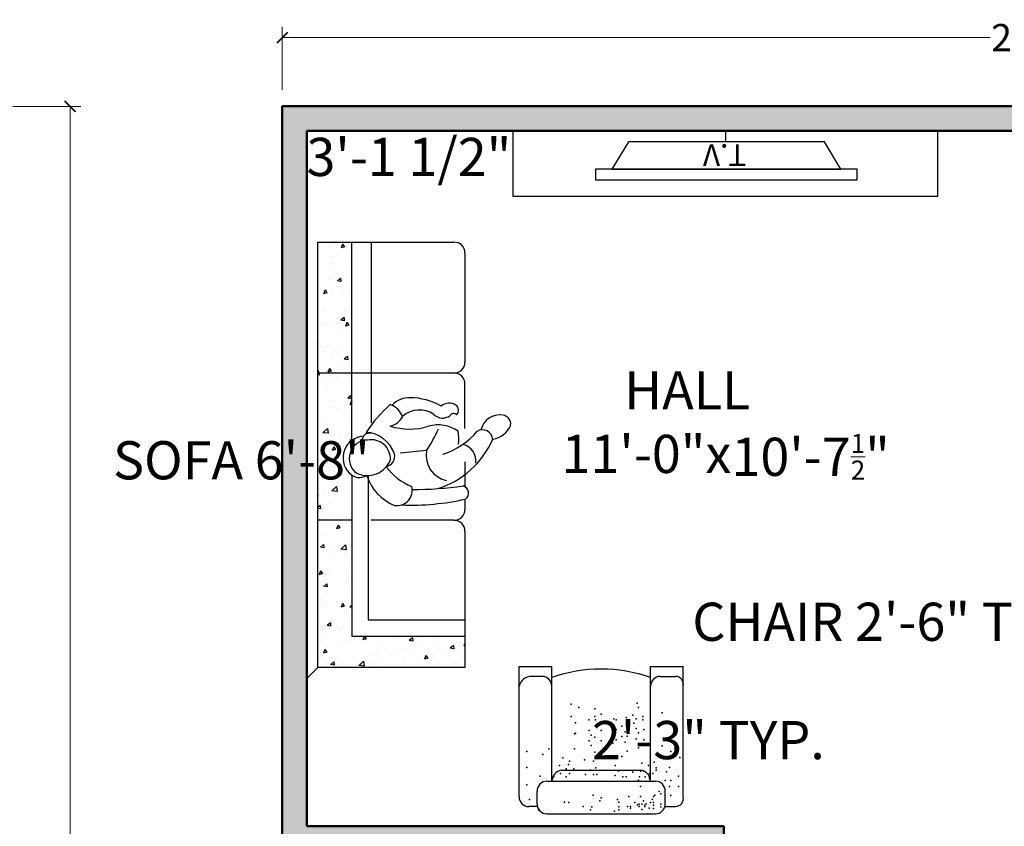
# Model space of a CAD drawing. Units: inches. Extents: x 4508 to 5907, y 877 to 1592.
# Tile 16 of 20: x 5203 to 5383, y 1443 to 1591. Entities that reach past the tile are written whole.
import ezdxf

# ---------------------------------------------------------------- set-up
doc = ezdxf.new("R2010")
doc.units = ezdxf.units.IN
doc.layers.get('DEFPOINTS').update_dxf_attribs({"color": 8})
for name, color, linetype, lineweight in [('A-ANNO-DIMS', 2, 'Continuous', 18), ('A-FURN', 24, 'Continuous', 18), ('A-WALL', 7, 'Continuous', 50), ('A-WALL-PATT', 8, 'Continuous', 13)]:
    doc.layers.add(name, color=color, linetype=linetype, lineweight=lineweight)
doc.layers.add('doors & windows', color=30, linetype='Continuous')
doc.layers.add('furniture', color=24, linetype='Continuous')
doc.styles.get("Standard").update_dxf_attribs({"font": 'arial.ttf'})
doc.dimstyles.new('details', dxfattribs={"dimtxt": 5, "dimasz": 2, "dimexe": 2, "dimexo": 3, "dimgap": 1, "dimtad": 0, "dimdec": 1, "dimzin": 0, "dimdsep": 46, "dimlunit": 4, "dimtxsty": 'Standard', "dimblk": 'ARCHTICK', "dimcen": 3, "dimclrd": 256, "dimclre": 256, "dimclrt": 256, "dimadec": 0, "dimazin": 0, "dimtfac": 0.5, "dimtdec": 1, "dimtofl": 0, "dimtmove": 0, "dimatfit": 3, "dimldrblk": 'CLOSEDBLANK', "dimfxl": 2, "dimtolj": 1, "dimtzin": 0, "dimlwd": -1, "dimlwe": -1, "dimarcsym": 0})
doc.dimstyles.new('text', dxfattribs={"dimtxt": 7, "dimasz": 0, "dimexe": 3, "dimexo": 3, "dimgap": 0, "dimtad": 1, "dimtih": 1, "dimtoh": 1, "dimzin": 3, "dimdsep": 46, "dimlunit": 4, "dimtxsty": 'Standard', "dimblk": 'CLOSEDBLANK', "dimcen": 3, "dimse1": 1, "dimse2": 1, "dimsd1": 1, "dimsd2": 1, "dimclrd": 256, "dimclre": 256, "dimclrt": 256, "dimadec": 0, "dimazin": 0, "dimtfac": 0.5, "dimtofl": 0, "dimtmove": 0, "dimatfit": 3, "dimfxl": 3, "dimtolj": 1, "dimtzin": 0, "dimlwd": -1, "dimlwe": -1, "dimarcsym": 0})

# ---------------------------------------------------------------- blocks, each defined once
blk = doc.blocks.new('_ArchTick')
at = {"color": 0, "linetype": 'ByBlock', "const_width": 0.15}
blk.add_lwpolyline([(-0.5, -0.5), (0.5, 0.5)], dxfattribs=at)
blk = doc.blocks.new('*D77')
at = {"layer": 'A-ANNO-DIMS', "color": 0, "transparency": 16777216}
for p, q in [((5201.49, 1574.7), (5213.97, 1574.7)), ((5211.97, 1574.7), (5211.97, 1255.95)), ((5211.97, 926.7), (5211.97, 1245.46)), ((5201.49, 926.7), (5213.97, 926.7))]:
    blk.add_line(p, q, dxfattribs=at)
at = {"layer": 'DEFPOINTS', "color": 0, "transparency": 16777216}
for p in [(5198.49, 1574.7), (5211.97, 1574.7), (5198.49, 926.7)]:
    blk.add_point(p, dxfattribs=at)
at = {"layer": 'A-ANNO-DIMS', "color": 0, "transparency": 16777216, "xscale": 2, "yscale": 2, "zscale": 2}
for p, rotation in [((5211.97, 1574.7), 90), ((5211.97, 926.7), 270)]:
    blk.add_blockref('_ArchTick', p, dxfattribs=dict(at, rotation=rotation))
at = {"layer": 'A-ANNO-DIMS', "color": 0, "transparency": 16777216, "insert": (5211.97, 1250.7), "char_height": 5, "attachment_point": 5, "rotation": 90}
blk.add_mtext("\\A1;54'", dxfattribs=at)
blk = doc.blocks.new('_ClosedBlank')
at = {"color": 0, "lineweight": -2}
for p, q in [((-1, 0.167), (0, 0)), ((-1, 0.167), (-1, -0.167)), ((0, 0), (-1, -0.167))]:
    blk.add_line(p, q, dxfattribs=at)
blk = doc.blocks.new('MAN')
at = {"layer": 'doors & windows'}
blk.add_line((1.3, -9.85), (0.89, -5.45), dxfattribs=at)
for centre, radius, start, end in [((0.1, 0.48), 3.6, 2.8928, 134.5528), ((-0.81, 1.3), 2.37, 132.7993, 210.1219), ((1.3, 0.05), 4.16, 155.2349, 248.5051), ((0, 0), 3.06, 359.7942, 144.0351), ((-0.36, -7.56), 8.07, 108.0153, 157.5724), ((-0.98, 0.55), 5.34, 289.2819, 356.6237), ((2.86, -0.44), 1.38, 352.7443, 87.7525), ((-8.99, -19.77), 24.04, 41.647, 56.3067), ((-0.1, -0.61), 3.22, 267.7788, 10.6507), ((4.14, -10.82), 9.46, 125.6851, 158.6987), ((0.38, -2.75), 1.79, 192.3382, 283.0231), ((-5.32, -4.92), 2.54, 170.002, 284.7527), ((15.87, -7.04), 10.97, 162.7002, 196.7262), ((8.59, -3.01), 3.29, 193.5598, 239.9446), ((5.83, -2.73), 3.32, 289.6374, 341.2911), ((6.12, -7.03), 4.01, 358.2671, 46.939), ((34.75, -7.19), 42.53, 177.9613, 192.4551), ((3.84, -8.67), 4.24, 325.4363, 41.8446), ((54.76, -7.35), 59.95, 180.1044, 188.2297), ((-0.78, -6.94), 10.91, 330.7562, 358.8997), ((0.5, -14.05), 4.27, 79.2575, 168.509), ((16.49, 13.41), 27.78, 236.8487, 245.427), ((-0.19, -11.81), 5.78, 325.2412, 16.1794), ((8.85, -12.54), 2.12, 136.0875, 215.1077), ((9.03, -7.36), 14.72, 197.1765, 246.7641), ((12.84, -8.62), 12.77, 197.9012, 229.3504), ((7.06, -13.61), 2.15, 328.4119, 38.6474), ((6.8, -14.37), 0.689, 315.9836, 61.7947), ((8.05, -14.12), 1.05, 224.0636, 323.687), ((-5.78, -15.61), 1.25, 217.214, 345.0614), ((-0.4, -15.27), 2.81, 261.6005, 345.5998), ((3.21, -8.72), 6.53, 262.8142, 281.931), ((3.09, -19.2), 1.68, 274.444, 31.8659), ((4.09, -22.01), 3.16, 349.15, 77.9716), ((6.99, -20.36), 3.8, 187.9766, 248.0432), ((5.75, -22.44), 1.45, 262.6631, 353.5986)]:
    blk.add_arc(centre, radius, start, end, dxfattribs=at)
blk = doc.blocks.new('sofa 2')
at = {"layer": 'furniture', "ltscale": 0.5}
h = blk.add_hatch(dxfattribs=at)
h.set_pattern_fill('AR-CONC', color=256, angle=450, style=0)
h.set_pattern_definition([(40, (-1099.1507, 871.655), (-0.627521, 7.172602), [0.75, -8.25]), (95, (-1099.151, 871.655), (7.52192, -1.387513), [0.6, -6.6]), (349.5486, (-1099.203, 872.253), (6.894395, 5.785094), [0.637402, -7.01142]), (43.8158, (-1097.151, 871.655), (-1.65519, 10.67241), [1.125, -12.375]), (353.3644, (-1097.289, 872.544), (9.74118, 9.34663), [0.9561, -10.51713]), (98.8158, (-1097.151, 871.655), (9.74119, 9.34662), [0.9, -9.9]), (69, (-1097.6507, 872.655), (-4.02619, 5.96907), [0.75, -8.25]), (124, (-1097.651, 872.655), (7.2515, 2.433153), [0.6, -6.6]), (18.5486, (-1097.986, 873.1524), (3.225305, 8.402226), [0.637402, -7.01142]), (52.5, (-1099.1507, 871.655), (3.3289385, 0.1215986), [0, -6.52, 0, -6.7, 0, -6.625]), (82.5, (-1099.1507, 871.655), (3.944117, 2.630695), [0, -3.82, 0, -6.37, 0, -2.525]), (122.5, (-1099.1507, 869.425), (-0.2255487, 5.3382244), [0, -2.5, 0, -7.8, 0, -10.35]), (132.5, (-1099.1507, 868.425), (1.00105, 5.831862), [0, -3.25, 0, -5.18, 0, -7.35])])
h.paths.add_polyline_path([(-8.27, -37.7, 0.168872), (-7.9, -36.76, 0.613808), (-6.95, -30.77, 0.074869), (-8.27, -30.38), (-8.27, -29), (-2, -29), (-2, -56), (-8.27, -56)])
h.paths.add_polyline_path([(-8.27, -7.77), (-29, -7.77), (-29, -2), (-2, -2), (-2, -29), (-8.27, -29)])
h.paths.add_polyline_path([(-8.27, -80), (-2, -80), (-2, -56), (-8.27, -56)])
at = {"layer": 'furniture'}
for p, q in [((-2, -2), (0, 0)), ((-29, -2), (-2, -2)), ((-29, -27), (-29, -2)), ((-2, -2), (-2, -80)), ((-8.27, -7.77), (-29, -7.77)), ((-8.27, -37.27), (-8.27, -7.77)), ((-11.27, -10.77), (-29, -10.77)), ((-11.27, -37.27), (-11.27, -10.77)), ((-27, -29), (-11.8, -29)), ((-8.27, -29), (-2, -29)), ((-29, -32.87), (-29, -31)), ((-29, -39.74), (-29, -35.16)), ((-8.27, -37.7), (-8.27, -37.7)), ((-8.27, -43.66), (-8.27, -80)), ((-29, -45.8), (-29, -54)), ((-11.8, -80), (-11.8, -46.89)), ((-27, -56), (-2, -56)), ((-29, -78), (-29, -58)), ((-2, -80), (-27, -80))]:
    blk.add_line(p, q, dxfattribs=at)
for centre, start, end in [((-27, -27), 180, 270), ((-27, -31), 90, 180), ((-27, -54), 180, 270), ((-27, -58), 90, 180), ((-27, -78), 180, 270)]:
    blk.add_arc(centre, 2, start, end, dxfattribs=at)
at = {"xscale": 1.099999999999999, "yscale": 1.099999999999999, "zscale": 1.099999999999999, "rotation": 270}
blk.add_blockref('MAN', (-11.13, -40.34), dxfattribs=at)
blk = doc.blocks.new('*D82')
at = {"layer": 'DEFPOINTS', "color": 0, "transparency": 16777216}
for p in [(5255.4, 1510.81), (5387.4, 1507.41), (5387.4, 1493.7)]:
    blk.add_point(p, dxfattribs=at)
at = {"layer": 'A-ANNO-DIMS', "color": 0, "transparency": 16777216, "insert": (5317.71, 1516.81), "char_height": 7, "width": 116.2892, "attachment_point": 5}
blk.add_mtext('\\A1;       HALL\\P11\'-0"x', dxfattribs=at)
blk = doc.blocks.new('*D83')
at = {"layer": 'DEFPOINTS', "color": 0, "transparency": 16777216}
for p in [(5332.19, 1570.2), (5347.84, 1570.2), (5313.91, 1442.7)]:
    blk.add_point(p, dxfattribs=at)
at = {"layer": 'A-ANNO-DIMS', "color": 0, "transparency": 16777216, "insert": (5347.84, 1510.45), "char_height": 7, "attachment_point": 5}
blk.add_mtext('\\A1;10\'-7{\\H0.5x;\\S1/2;}"', dxfattribs=at)
blk = doc.blocks.new('tv')
at = {"layer": 'furniture'}
blk.add_line((0, 0), (2, 0), dxfattribs=at)
for points in [[(0, -39), (12, -39), (12, 39), (0, 39)], [(7, 24.19), (7, -23.81), (9, -23.81), (9, 24.19), (7, 24.19)]]:
    blk.add_lwpolyline(points, dxfattribs=at)
blk.add_lwpolyline([(7, -20.81), (7, 21.19), (2, 18.19), (2, -17.81)], close=True, dxfattribs=at)
blk.add_text('T.V', height=4, rotation=270, dxfattribs=at).set_placement((2.46, 3.81))
blk = doc.blocks.new('sofa')
at = {"layer": 'furniture'}
for p, q in [((3.13, 15.05), (27, 15.05)), ((27, 15.05), (27, 9.05)), ((1.33, 11.75), (1.33, 13.25)), ((25.2, 10.85), (25.2, 12.75)), ((1.8, 11.75), (4.13, 11.75)), ((0, 9.95), (0, -9.95)), ((6, 9.95), (6, -9.95)), ((6, 9.05), (27, 9.05)), ((8, 7.25), (8, -7.25)), ((8, 4.04), (8, 3.89)), ((6.03, -9.05), (27, -9.05)), ((27, -9.05), (27, -15.05)), ((1.33, -11.75), (1.33, -13.65)), ((1.8, -11.75), (4.13, -11.75)), ((25.2, -10.85), (25.2, -13.65)), ((3.13, -15.05), (27, -15.05))]:
    blk.add_line(p, q, dxfattribs=at)
for centre, radius, start, end in [((3.13, 13.25), 1.8, 90, 180), ((22.91, 12.82), 2.29, 358.3453, 77.7487), ((1.8, 9.95), 1.8, 90, 180), ((1.8, 9.95), 1.8, 90, 180), ((4.14, 9.89), 1.86, 1.747, 90.2901), ((4.14, 9.89), 1.86, 1.747, 90.2901), ((23.4, 10.85), 1.8, 270, 0), ((5.91, 6.93), 2.12, 8.589, 87.4366), ((-0.79, 0), 27.33, 340.6621, 19.3379), ((5.96, -6.99), 2.06, 272.0036, 352.7589), ((1.8, -9.95), 1.8, 180, 270), ((4.14, -9.89), 1.86, 269.7099, 358.253), ((23.4, -10.85), 1.8, 0, 90), ((2.83, -13.59), 1.5, 182.4941, 281.7559), ((23.7, -13.59), 1.5, 258.2441, 357.5059)]:
    blk.add_arc(centre, radius, start, end, dxfattribs=at)
for p in [(2.64, 13.13), (5.3, 13.66), (8.48, 13.66), (11.4, 13.66), (0.72, 11.51), (6.89, 11.2), (10.87, 10.67), (11.93, 9.61), (6.8, 8.68), (7.42, 7.45), (8.85, 7.66), (2.09, 5.95), (2.11, 6.75), (6.8, 6.43), (7.42, 5.82), (8.24, 6.43), (9.05, 6.02), (9.67, 5.82), (10.28, 7.04), (17.83, 5.52), (20.08, 5.52), (8.24, 5), (11.92, 4.9), (14.64, 4.9), (14.78, 4.7), (16.69, 4.7), (19.47, 4.09), (0.72, 1.97), (1.32, 3.3), (7.21, 2.86), (8.03, 2.04), (9.87, 3.06), (12.53, 1.84), (13.35, 2.21), (14.44, 1.84), (15.26, 2.21), (17.21, 2.25), (1.3, 1.71), (2.38, 0.24), (3.44, 1.44), (7.21, 1.39), (7.21, 0.82), (8.44, 0.98), (9.67, 1.43), (10.49, 0.98), (11.31, 1.19), (13.35, 0.01), (14.03, 1.19), (15.26, 0.01), (17.24, 1.02), (17.85, 1.19), (19.26, 1.19), (2.91, -0.01), (18.24, -0.03), (0.5, -2.45), (0.72, -3.25), (1.26, -3.25), (2.11, -3.25), (2.64, -2.98), (7.01, -2.55), (7.83, -3.16), (8.85, -2.55), (12.94, -2.14), (13.56, -2.75), (14.85, -2.14), (15.46, -2.75), (17.21, -2.75), (17.44, -2.34), (1.03, -5.36), (1.32, -5.36), (1.36, -4.83), (3.17, -5.1), (6.8, -3.98), (6.8, -4.59), (10.49, -3.77), (11.51, -4.79), (13.15, -4.38), (14.17, -3.77), (14.23, -4.79), (15.05, -4.38), (16.07, -3.77), (16.8, -4.79), (17.65, -4.59), (1.36, -6.95), (1.62, -6.69), (1.79, -6.95), (2.05, -6.16), (3.17, -7.22), (5.03, -7.22), (6.19, -6.84), (6.8, -7.04), (7.62, -5.82), (12.12, -6.84), (13.76, -6.43), (14.85, -6.84), (15.66, -6.43), (16.6, -6.02), (17.44, -6.43), (18.06, -5.82), (19.47, -6.84), (20.28, -6.63), (-0.03, -8.54), (0.77, -7.48), (1.03, -8.81), (1.36, -8.01), (1.56, -8.01), (1.79, -7.48), (1.85, -8.28), (2.38, -7.75), (6.39, -8.88), (6.8, -8.06), (7.42, -8.88), (7.83, -7.25), (7.83, -7.86), (8.85, -8.68), (9.26, -7.45), (13.56, -7.86), (15.46, -7.86), (17.24, -7.65), (17.83, -7.65), (0.99, -9.6), (1.58, -9.6), (2.05, -9.07), (2.09, -9.6), (2.64, -9.34), (3.17, -9.6), (3.44, -9.87), (4.09, -10.66), (7.42, -9.49), (8.03, -10.11), (8.44, -10.11), (9.46, -9.7), (1.3, -10.93), (1.79, -10.93), (3.64, -10.93), (5.03, -12.52), (6.09, -11.72), (7.69, -11.99), (8.48, -12.52), (12.46, -11.19), (18.51, -11.19), (3.38, -12.78), (5.03, -14.17), (6.09, -12.78), (6.89, -14.17), (10.34, -14.44), (11.4, -12.78)]:
    blk.add_point(p, dxfattribs=at)
blk = doc.blocks.new('*D112')
at = {"layer": 'A-ANNO-DIMS', "color": 0, "transparency": 16777216}
for p, q in [((5250.9, 1577.7), (5250.9, 1589.3)), ((5529.9, 1577.7), (5529.9, 1589.3)), ((5250.9, 1587.3), (5380.77, 1587.3)), ((5529.9, 1587.3), (5400.03, 1587.3))]:
    blk.add_line(p, q, dxfattribs=at)
at = {"layer": 'DEFPOINTS', "color": 0, "transparency": 16777216}
for p in [(5529.9, 1587.3), (5250.9, 1574.7), (5529.9, 1574.7)]:
    blk.add_point(p, dxfattribs=at)
at = {"layer": 'A-ANNO-DIMS', "color": 0, "transparency": 16777216, "xscale": 2, "yscale": 2, "zscale": 2, "rotation": 180}
blk.add_blockref('_ArchTick', (5250.9, 1587.3), dxfattribs=at)
at = {"layer": 'A-ANNO-DIMS', "color": 0, "transparency": 16777216, "xscale": 2, "yscale": 2, "zscale": 2}
blk.add_blockref('_ArchTick', (5529.9, 1587.3), dxfattribs=at)
at = {"layer": 'A-ANNO-DIMS', "color": 0, "transparency": 16777216, "insert": (5390.4, 1587.3), "char_height": 5, "attachment_point": 5}
blk.add_mtext('\\A1;23\'-3"', dxfattribs=at)
blk = doc.blocks.new('*D174')
at = {"layer": 'DEFPOINTS', "color": 0, "transparency": 16777216}
for p in [(5294.35, 1476.58), (5294.35, 1472.05), (5324.54, 1472.05)]:
    blk.add_point(p, dxfattribs=at)
at = {"layer": 'A-ANNO-DIMS', "transparency": 16777216, "insert": (5362.41, 1480.2), "char_height": 7, "attachment_point": 5}
blk.add_mtext('\\A1;CHAIR 2\'-6" TYP.', dxfattribs=at)
blk = doc.blocks.new('*D175')
at = {"layer": 'DEFPOINTS', "color": 0, "transparency": 16777216}
for p in [(5324.54, 1472.05), (5329.07, 1472.05), (5324.54, 1444.96)]:
    blk.add_point(p, dxfattribs=at)
at = {"layer": 'A-ANNO-DIMS', "transparency": 16777216, "insert": (5329.07, 1458.51), "char_height": 7, "attachment_point": 5}
blk.add_mtext('\\A1;2\'-3" TYP.', dxfattribs=at)
blk = doc.blocks.new('*D178')
at = {"layer": 'DEFPOINTS', "color": 0, "transparency": 16777216}
for p in [(5255.4, 1549.81), (5243.4, 1469.81), (5255.4, 1469.81)]:
    blk.add_point(p, dxfattribs=at)
at = {"layer": 'A-ANNO-DIMS', "transparency": 16777216, "insert": (5243.4, 1509.81), "char_height": 7, "attachment_point": 5}
blk.add_mtext('\\A1;SOFA 6\'-8"', dxfattribs=at)
blk = doc.blocks.new('*D179')
at = {"layer": 'DEFPOINTS', "color": 0, "transparency": 16777216}
for p in [(5255.4, 1561.81), (5255.4, 1549.81), (5292.85, 1549.81)]:
    blk.add_point(p, dxfattribs=at)
at = {"layer": 'A-ANNO-DIMS', "transparency": 16777216, "insert": (5274.13, 1565.43), "char_height": 7, "attachment_point": 5}
blk.add_mtext('\\A1;3\'-1 1/2"', dxfattribs=at)

msp = doc.modelspace()

# ---------------------------------------------------------------- hatches: boundary and pattern name
at = {"layer": 'A-WALL-PATT'}
h = msp.add_hatch(color=256, dxfattribs=at)
h.dxf.hatch_style = 1
h.paths.add_polyline_path([(5529.903, 1303.204), (5388.02, 1303.204), (5388.02, 1294.204), (5391.903, 1294.204), (5391.903, 1205.704), (5396.403, 1205.704), (5396.403, 1294.204), (5489.403, 1294.204), (5489.403, 1256.139), (5493.903, 1256.139), (5493.903, 1294.204), (5529.903, 1294.204)], flags=17)
h.paths.add_polyline_path([(5346.02, 1303.204), (5322.903, 1303.204), (5322.903, 1321.388), (5313.903, 1321.388), (5313.903, 1303.204), (5259.903, 1303.204), (5259.903, 1381.204), (5313.903, 1381.204), (5313.903, 1359.674), (5322.903, 1359.674), (5322.903, 1381.204), (5338.979, 1381.204), (5338.979, 1390.204), (5331.903, 1390.204), (5331.903, 1442.704), (5255.403, 1442.704), (5255.403, 1570.204), (5387.403, 1570.204), (5387.403, 1541.271), (5391.903, 1541.271), (5391.903, 1570.204), (5483.403, 1570.204), (5483.403, 1498.204), (5391.903, 1498.204), (5391.903, 1509.559), (5387.403, 1509.559), (5387.403, 1390.204), (5380.979, 1390.204), (5380.979, 1381.204), (5387.403, 1381.204), (5529.903, 1381.204), (5529.903, 1498.204), (5487.903, 1498.204), (5487.903, 1570.204), (5529.903, 1570.204), (5529.903, 1574.704), (5250.903, 1574.704), (5250.903, 991.204), (5310.903, 991.204), (5310.903, 926.704), (5529.903, 926.704), (5529.903, 1210.204), (5525.403, 1210.204), (5525.403, 1103.704), (5499.903, 1103.704), (5499.903, 1210.204), (5493.903, 1210.204), (5493.903, 1256.139), (5489.403, 1256.139), (5489.403, 1210.204), (5461.584, 1210.204), (5461.584, 1205.704), (5495.403, 1205.704), (5495.403, 1103.704), (5436.903, 1103.704), (5436.903, 1051.204), (5391.954, 1051.204), (5391.954, 1103.03), (5391.954, 1107.53), (5255.403, 1108.204), (5255.403, 1294.204), (5346.02, 1294.204)])
h.paths.add_polyline_path([(5255.403, 1390.204), (5255.403, 1398.204), (5255.403, 1438.204), (5257.903, 1438.204), (5258.903, 1438.204), (5327.403, 1438.204), (5327.403, 1390.204), (5325.903, 1390.204)], flags=16)
h.paths.add_polyline_path([(5288.757, 1390.704), (5288.757, 1390.204), (5292.173, 1390.204), (5292.173, 1390.704)], flags=0)
h.paths.add_polyline_path([(5289.965, 1391.606), (5289.965, 1396.645), (5289.903, 1396.645), (5289.903, 1397.319), (5288.849, 1398.862), (5288.849, 1398.8), (5288.983, 1398.748), (5288.983, 1399.204), (5289.091, 1399.204), (5292.081, 1399.204), (5292.081, 1398.665), (5291.946, 1398.665), (5291.027, 1397.319), (5291.027, 1396.645), (5290.965, 1396.645), (5290.965, 1391.606)], flags=0)
h.paths.add_polyline_path([(5288.849, 1399.069, 2.6374395), (5289.056, 1398.835), (5289.117, 1399.087, 0.9346155)], flags=0)
h.paths.add_polyline_path([(5290.061, 1398.665), (5290.061, 1399.204), (5290.038, 1398.975)], flags=0)
h.paths.add_polyline_path([(5291.946, 1398.934, -1), (5291.946, 1398.665)], flags=0)
h.paths.add_polyline_path([(5289.414, 1398.967), (5289.414, 1399.204), (5289.63, 1399.204), (5289.63, 1398.363), (5290.051, 1397.184), (5290.76, 1397.184), (5290.869, 1398.665), (5290.869, 1399.204), (5290.815, 1398.665), (5290.815, 1399.204), (5291.462, 1399.204), (5291.462, 1398.816), (5290.879, 1397.184), (5290.051, 1397.184)], flags=0)
h.paths.add_polyline_path([(5273.903, 1392.056), (5269.591, 1392.056, 0.0901028), (5265.544, 1392.842), (5265.511, 1392.034, -0.3516542), (5265.903, 1391.546, -1), (5264.903, 1391.546, -0.3042165), (5265.213, 1392.008), (5265.167, 1392.84, 0.0880132), (5261.215, 1392.056), (5256.903, 1392.056), (5256.903, 1398.704, -0.4142136), (5259.403, 1401.204), (5271.403, 1401.204, -0.4142136), (5273.903, 1398.704)], flags=0)
h.paths.add_polyline_path([(5263.726, 1395.073, -1), (5267.08, 1395.073, -1)], flags=0)
h.paths.add_polyline_path([(5264.434, 1395.073, -0.695521), (5265.153, 1395.073, -1.1408699), (5265.403, 1395.585, -0.7522125), (5265.403, 1396.25, 0.3674806)], flags=0)
h.paths.add_polyline_path([(5265.153, 1394.399, -1), (5265.653, 1394.399, -1)], flags=0)
h.paths.add_polyline_path([(5265.905, 1395.077, -1), (5266.405, 1395.077, -1)], flags=0)
h.paths.add_polyline_path([(5307.994, 1403.113, -1), (5307.994, 1417.295), (5318.794, 1417.295, -0.4142136), (5319.794, 1416.295), (5320.794, 1416.295, -0.4142136), (5321.794, 1417.295), (5324.903, 1417.295, -0.4142136), (5325.903, 1416.295), (5325.903, 1404.113, -0.4142136), (5324.903, 1403.113), (5321.794, 1403.113, -0.4142136), (5320.794, 1404.113), (5319.794, 1404.113, -0.4142136), (5318.794, 1403.113)], flags=0)
h.paths.add_polyline_path([(5307.836, 1405.113, -1), (5307.836, 1415.295), (5315.591, 1415.295, -0.4142136), (5317.532, 1413.353), (5317.532, 1407.054, -0.4142136), (5315.591, 1405.113)], flags=0)
h.paths.add_polyline_path([(5312.032, 1408.204, -1), (5312.032, 1412.204), (5315.032, 1412.204, -0.4142136), (5316.032, 1411.204), (5316.032, 1409.204, -0.4142136), (5315.032, 1408.204)], flags=0)
h.paths.add_polyline_path([(5391.903, 1385.704), (5391.903, 1493.704), (5525.403, 1493.704), (5525.403, 1385.704)], flags=16)
h.paths.add_polyline_path([(5422.641, 1390.704), (5422.641, 1465.704, -0.9426302), (5422.641, 1467.704), (5494.547, 1467.704, -1), (5494.665, 1465.704), (5494.665, 1390.704, -0.9426302), (5494.665, 1388.704), (5422.759, 1388.704, -1)], flags=0)
h.paths.add_polyline_path([(5427.52, 1395.749, -0.0238564), (5427.614, 1403.949, 0.0884332), (5427.476, 1405.056, 0.0506693), (5427.273, 1405.463, -0.8716827), (5427.713, 1405.835, 0.0268855), (5431.815, 1405.361, 0.0306964), (5436.289, 1405.361, -0.0263641), (5445.798, 1405.259, 0.075811), (5450.408, 1405.53, 0.0687062), (5454.457, 1405.903, -1.0086747), (5454.781, 1405.482, 0.0692081), (5454.389, 1400.959, -0.0519468), (5454.356, 1394.996, 0.1195012), (5454.627, 1392.895, 0.0143508), (5454.796, 1392.489, -0.6962059), (5454.42, 1392.118, 0.1574808), (5448.747, 1392.794, -0.025536), (5432.749, 1392.774, 0.0920085), (5427.781, 1392.048, -0.9384848), (5427.137, 1392.455, 0.0063894), (5427.314, 1392.79, 0.0472995)], flags=0)
h.paths.add_polyline_path([(5426.125, 1411.372, 0.0617649), (5428.641, 1412.201), (5428.641, 1465.704), (5488.665, 1465.704), (5488.665, 1412.363, 0.2363822), (5467.6, 1412.052, -0.2252042)], flags=0)
h.paths.add_polyline_path([(5391.903, 1490.204), (5391.903, 1491.204), (5422.903, 1491.204), (5422.903, 1490.204)], flags=0)
h.paths.add_polyline_path([(5462.545, 1392.771, 0.1270318), (5462.866, 1394.996, -0.0519468), (5462.832, 1400.959, 0.0692081), (5462.441, 1405.482, -1.0086747), (5462.765, 1405.903, 0.0857004), (5471.424, 1405.259, -0.0263641), (5480.932, 1405.361, 0.0306964), (5485.407, 1405.361, 0.0268855), (5489.509, 1405.835, -0.8716827), (5489.949, 1405.463, 0.0506693), (5489.746, 1405.056, 0.0884332), (5489.608, 1403.949, -0.0238564), (5489.702, 1395.749, 0.0472995), (5489.908, 1392.79, 0.0063894), (5490.085, 1392.455, -0.9384848), (5489.441, 1392.048, 0.0920085), (5484.473, 1392.774, -0.025536), (5468.475, 1392.794, 0.1574808), (5462.802, 1392.118, -0.6962059), (5462.426, 1392.489, 0.0100173), (5462.546, 1392.771)], flags=0)
h.paths.add_polyline_path([(5387.454, 1103.03), (5387.454, 1100.53), (5387.454, 1099.53), (5387.454, 995.03), (5387.454, 991.204), (5391.954, 991.204), (5391.954, 1046.704), (5525.403, 1046.704), (5525.403, 931.182), (5391.954, 930.53), (5391.954, 960.53), (5387.454, 960.53), (5387.454, 930.53), (5315.403, 930.53), (5315.403, 991.204), (5323.403, 991.204), (5387.454, 991.204), (5387.454, 995.03), (5255.403, 995.704), (5255.403, 1103.704)], flags=16)
h.paths.add_polyline_path([(5379.264, 1062.889), (5379.264, 1060.156), (5385.764, 1061.889, -0.4526903), (5385.764, 1059.889), (5379.264, 1059.889), (5379.264, 1055.156), (5385.764, 1056.889, -0.4526903), (5385.764, 1054.889), (5379.264, 1054.889), (5379.264, 1050.156), (5385.764, 1051.889, -0.4526903), (5385.764, 1049.889), (5379.264, 1049.889), (5379.264, 1010.156), (5385.764, 1011.889, -0.4526903), (5385.764, 1009.889), (5379.264, 1009.889), (5379.264, 1005.156), (5385.764, 1006.889, -0.4526903), (5385.764, 1004.889), (5379.264, 1004.889), (5379.264, 1000.156), (5385.764, 1001.889, -0.4526903), (5385.764, 999.889), (5378.264, 999.889), (5370.764, 997.889, -0.6674863), (5370.764, 999.889), (5377.264, 999.889), (5377.264, 1004.623), (5370.764, 1002.889, -0.6674863), (5370.764, 1004.889), (5377.264, 1004.889), (5377.264, 1009.623), (5370.764, 1007.889, -0.6674863), (5370.764, 1009.889), (5377.264, 1009.889), (5377.264, 1049.623), (5370.764, 1047.889, -0.6674863), (5370.764, 1049.889), (5377.264, 1049.889), (5377.264, 1054.623), (5370.764, 1052.889, -0.6674863), (5370.764, 1054.889), (5377.264, 1054.889), (5377.264, 1059.623), (5370.764, 1057.889, -0.6674863), (5370.764, 1059.889), (5377.264, 1059.889), (5377.264, 1062.889)], flags=0)
h.paths.add_polyline_path([(5287.641, 1000.704), (5359.665, 1000.704), (5359.665, 1018.212, 0.3202856), (5332.6, 1022.052, -0.246494), (5287.641, 1023.128)], flags=0)
h.paths.add_polyline_path([(5359.547, 1077.704, -1), (5359.665, 1075.704), (5353.665, 1075.704), (5353.665, 1063.704), (5293.641, 1063.704), (5293.641, 1075.704), (5287.759, 1075.704, -1), (5287.641, 1077.704)], flags=0)
h.paths.add_polyline_path([(5441.403, 1099.204), (5525.403, 1099.204), (5525.403, 1051.204), (5441.403, 1051.204), (5441.403, 1059.204)], flags=16)
h.paths.add_polyline_path([(5441.403, 1096.704), (5466.403, 1096.704), (5466.403, 1095.704), (5441.403, 1095.704)], flags=0)
h.paths.add_polyline_path([(5445.403, 1062.204), (5457.403, 1062.204, -0.4142136), (5459.903, 1059.704), (5459.903, 1053.056), (5455.591, 1053.056, 0.0901028), (5451.544, 1053.842), (5451.511, 1053.034, -0.3516542), (5451.903, 1052.546, -1), (5450.903, 1052.546, -0.3042165), (5451.213, 1053.008), (5451.167, 1053.84, 0.0880132), (5447.215, 1053.056), (5442.903, 1053.056), (5442.903, 1059.704, -0.4142136)], flags=0)
h.paths.add_polyline_path([(5453.08, 1056.073, -1), (5449.726, 1056.073, -1)], flags=0)
h.paths.add_polyline_path([(5292.713, 1015.835, 0.0268855), (5296.815, 1015.361, 0.0306964), (5301.289, 1015.361, -0.0263641), (5310.798, 1015.259, 0.075811), (5315.408, 1015.53, 0.0687062), (5319.457, 1015.903, -1.0086747), (5319.781, 1015.482, 0.0692081), (5319.389, 1010.959, -0.0519468), (5319.356, 1004.996, 0.1195012), (5319.627, 1002.895, 0.0143508), (5319.796, 1002.489, -0.6962059), (5319.42, 1002.118, 0.1574808), (5313.747, 1002.794, -0.025536), (5297.749, 1002.774, 0.0920085), (5292.781, 1002.048, -0.9384848), (5292.137, 1002.455, 0.0063894), (5292.314, 1002.79, 0.0472995), (5292.52, 1005.749, -0.0238564), (5292.614, 1013.949, 0.0884332), (5292.476, 1015.056, 0.0506693), (5292.273, 1015.463, -0.8716827)], flags=0)
h.paths.add_polyline_path([(5450.434, 1056.073, -0.695521), (5451.153, 1056.073, -1.1408699), (5451.403, 1056.585, -0.7522125), (5451.403, 1057.25, 0.3674806)], flags=0)
h.paths.add_polyline_path([(5327.765, 1015.903, 0.0857004), (5336.424, 1015.259, -0.0263641), (5345.932, 1015.361, 0.0306964), (5350.407, 1015.361, 0.0268855), (5354.509, 1015.835, -0.8716827), (5354.949, 1015.463, 0.0506693), (5354.746, 1015.056, 0.0884332), (5354.608, 1013.949, -0.0238564), (5354.702, 1005.749, 0.0472995), (5354.908, 1002.79, 0.0063894), (5355.085, 1002.455, -0.9384848), (5354.441, 1002.048, 0.0920085), (5349.473, 1002.774, -0.025536), (5333.475, 1002.794, 0.1574808), (5327.802, 1002.118, -0.6962059), (5327.426, 1002.489, 0.0100173), (5327.546, 1002.771), (5327.545, 1002.771, 0.1270318), (5327.866, 1004.996, -0.0519468), (5327.832, 1010.959, 0.0692081), (5327.441, 1015.482, -1.0086747)], flags=0)
h.paths.add_polyline_path([(5452.405, 1056.077, -1), (5451.905, 1056.077, -1)], flags=0)
h.paths.add_polyline_path([(5451.653, 1055.399, -1), (5451.153, 1055.399, -1)], flags=0)
h.paths.add_polyline_path([(5472.958, 1051.704), (5472.958, 1051.204), (5476.374, 1051.204), (5476.374, 1051.704)], flags=0)
h.paths.add_polyline_path([(5476.282, 1060.204), (5476.282, 1059.665), (5476.147, 1059.665), (5475.228, 1058.319), (5475.228, 1057.645), (5475.166, 1052.606), (5474.166, 1052.606), (5474.166, 1057.645), (5474.104, 1057.645), (5474.104, 1058.319), (5473.05, 1059.862), (5473.05, 1059.8), (5473.184, 1059.748), (5473.184, 1060.204), (5473.292, 1060.204)], flags=0)
h.paths.add_polyline_path([(5473.05, 1060.069, 2.6374395), (5473.257, 1059.835), (5473.318, 1060.087, 0.9346155)], flags=0)
h.paths.add_polyline_path([(5473.831, 1060.204), (5473.831, 1059.363), (5474.252, 1058.184), (5474.371, 1058.184), (5474.262, 1059.665), (5474.262, 1060.204)], flags=0)
h.paths.add_polyline_path([(5475.501, 1060.204), (5475.501, 1059.363), (5475.555, 1059.514), (5475.555, 1060.204)], flags=0)
h.paths.add_polyline_path([(5474.855, 1060.204), (5474.908, 1060.127), (5474.908, 1060.204), (5474.855, 1059.665)], flags=0)
h.paths.add_polyline_path([(5476.147, 1059.934, -1), (5476.147, 1059.665)], flags=0)
h.paths.add_polyline_path([(5474.693, 1060.204), (5475.178, 1059.511), (5475.178, 1060.204), (5475.285, 1059.934), (5475.285, 1060.204), (5475.178, 1059.665), (5475.178, 1060.204), (5475.07, 1059.665), (5475.07, 1060.204), (5474.962, 1059.665), (5474.962, 1060.204), (5474.693, 1059.306)], flags=0)
h.paths.add_polyline_path([(5474.747, 1060.204), (5474.37, 1059.45), (5474.37, 1060.204), (5474.424, 1060.096), (5474.424, 1060.204), (5474.747, 1059.665)], flags=0)
h.paths.add_polyline_path([(5476.04, 1059.665), (5476.04, 1060.204), (5476.094, 1059.665), (5476.094, 1060.204)], flags=0)
h.paths.add_polyline_path([(5505.994, 1082.295), (5516.794, 1082.295, -0.4142136), (5517.794, 1081.295), (5518.794, 1081.295, -0.4142136), (5519.794, 1082.295), (5522.903, 1082.295, -0.4142136), (5523.903, 1081.295), (5523.903, 1069.113, -0.4142136), (5522.903, 1068.113), (5519.794, 1068.113, -0.4142136), (5518.794, 1069.113), (5517.794, 1069.113, -0.4142136), (5516.794, 1068.113), (5505.994, 1068.113, -1)], flags=0)
h.paths.add_polyline_path([(5505.836, 1080.295), (5513.591, 1080.295, -0.4142136), (5515.532, 1078.353), (5515.532, 1072.054, -0.4142136), (5513.591, 1070.113), (5505.836, 1070.113, -1)], flags=0)
h.paths.add_polyline_path([(5520.403, 963.695), (5520.403, 1035.72), (5502.895, 1035.72, 0.3202856), (5499.055, 1008.654, -0.246494), (5497.978, 963.695)], flags=0)
h.paths.add_polyline_path([(5445.403, 1035.72), (5445.403, 1029.72), (5457.403, 1029.72), (5457.403, 969.695), (5445.403, 969.695), (5445.403, 963.814, -1), (5443.403, 963.695), (5443.403, 1035.602, -1)], flags=0)
h.paths.add_polyline_path([(5510.032, 1077.204), (5513.032, 1077.204, -0.4142136), (5514.032, 1076.204), (5514.032, 1074.204, -0.4142136), (5513.032, 1073.204), (5510.032, 1073.204, -1)], flags=0)
h.paths.add_polyline_path([(5317.255, 989.704), (5323.903, 989.704, -0.4142136), (5326.403, 987.204), (5326.403, 975.204, -0.4142136), (5323.903, 972.704), (5317.255, 972.704), (5317.255, 977.016, 0.0901028), (5318.041, 981.063), (5317.233, 981.096, -0.8964437), (5316.245, 981.204, -0.8220123), (5317.207, 981.394), (5318.04, 981.44, 0.0880132), (5317.255, 985.392)], flags=0)
h.paths.add_polyline_path([(5321.949, 981.204, -1), (5318.594, 981.204, -1)], flags=0)
h.paths.add_polyline_path([(5362.454, 988.03), (5387.454, 988.03), (5387.454, 990.53), (5391.954, 990.53), (5391.704, 988.289, -0.4090807), (5391.204, 987.78), (5391.204, 987.53), (5388.954, 987.53), (5388.954, 988.03), (5387.454, 988.03), (5387.454, 987.03), (5362.474, 987.03, 0.4025427), (5387.454, 963.03), (5388.954, 963.03), (5388.954, 963.53), (5391.195, 963.28, -0.4142136), (5391.704, 962.771), (5391.954, 960.53), (5391.954, 962.78), (5391.704, 962.78, 0.4090807), (5391.195, 963.28), (5388.954, 963.53), (5388.954, 963.03), (5387.454, 963.03, -0.4025427), (5362.474, 987.03), (5362.454, 987.03)], flags=0)
h.paths.add_polyline_path([(5321.285, 981.204, -0.6555366), (5320.522, 981.204, -1.1195284), (5320.275, 980.701, -1.3500746), (5320.279, 980.026, 0.3749463)], flags=0)
h.paths.add_polyline_path([(5320.022, 981.923, -1), (5320.522, 981.923, -1)], flags=0)
h.paths.add_polyline_path([(5319.348, 981.204, -1), (5319.848, 981.204, -1)], flags=0)
h.paths.add_polyline_path([(5507.157, 1030.662, -0.0238564), (5515.358, 1030.756, 0.0472995), (5518.317, 1030.962, 0.0063894), (5518.652, 1031.139, -0.9384848), (5519.059, 1030.495, 0.0920085), (5518.333, 1025.527, -0.025536), (5518.313, 1009.53, 0.1574808), (5518.989, 1003.857, -0.6962059), (5518.618, 1003.48, 0.0100173), (5518.335, 1003.601), (5518.335, 1003.6, 0.1270318), (5516.111, 1003.921, -0.0519468), (5510.148, 1003.887, 0.0692081), (5505.624, 1003.495, -1.0086747), (5505.204, 1003.819, 0.0857004), (5505.848, 1012.479, -0.0263641), (5505.746, 1021.987, 0.0306964), (5505.746, 1026.462, 0.0268855), (5505.272, 1030.563, -0.8716827), (5505.644, 1031.004, 0.0506693), (5506.051, 1030.801, 0.0884332)], flags=0)
h.paths.add_polyline_path([(5368.045, 945.621), (5378.845, 945.621, -0.4142136), (5379.845, 944.621), (5380.845, 944.621, -0.4142136), (5381.845, 945.621), (5384.954, 945.621, -0.4142136), (5385.954, 944.621), (5385.954, 932.439, -0.4142136), (5384.954, 931.439), (5381.845, 931.439, -0.4142136), (5380.845, 932.439), (5379.845, 932.439, -0.4142136), (5378.845, 931.439), (5368.045, 931.439, -1)], flags=0)
h.paths.add_polyline_path([(5327.31, 931.03), (5327.31, 930.53), (5330.726, 930.53), (5330.726, 931.03)], flags=0)
h.paths.add_polyline_path([(5330.634, 939.53), (5330.634, 938.991), (5330.499, 938.991), (5329.579, 937.645), (5329.579, 936.971), (5329.518, 936.971), (5329.518, 931.933), (5328.518, 931.933), (5328.518, 936.971), (5328.456, 936.971), (5328.456, 937.645), (5327.402, 939.189), (5327.402, 939.126), (5327.536, 939.074), (5327.536, 939.53), (5327.644, 939.53)], flags=0)
h.paths.add_polyline_path([(5327.402, 939.395, 2.6374395), (5327.609, 939.161), (5327.67, 939.414, 0.9346155)], flags=0)
h.paths.add_polyline_path([(5328.021, 939.142), (5328.021, 939.53), (5327.967, 939.53), (5327.967, 939.293)], flags=0)
h.paths.add_polyline_path([(5328.614, 939.53), (5328.614, 938.991), (5328.723, 937.51), (5329.313, 937.51), (5329.422, 938.991), (5329.422, 939.53), (5329.368, 938.991), (5329.368, 939.53)], flags=0)
h.paths.add_polyline_path([(5329.853, 939.53), (5329.853, 938.689), (5329.907, 938.84), (5329.907, 939.53)], flags=0)
h.paths.add_polyline_path([(5330.499, 939.261, -1), (5330.499, 938.991)], flags=0)
h.paths.add_polyline_path([(5367.887, 943.621), (5375.641, 943.621, -0.4142136), (5377.583, 941.68), (5377.583, 935.38, -0.4142136), (5375.641, 933.439), (5367.887, 933.439, -1)], flags=0)
h.paths.add_polyline_path([(5509.267, 947.14), (5509.267, 939.64), (5511.267, 932.14, -0.4526903), (5509.267, 932.14), (5509.267, 938.64), (5504.534, 938.64), (5506.267, 932.14, -0.4526903), (5504.267, 932.14), (5504.267, 938.64), (5499.534, 938.64), (5501.267, 932.14, -0.4526903), (5499.267, 932.14), (5499.267, 938.64), (5459.534, 938.64), (5461.267, 932.14, -0.4526903), (5459.267, 932.14), (5459.267, 938.64), (5454.534, 938.64), (5456.267, 932.14, -0.4526903), (5454.267, 932.14), (5454.267, 938.64), (5449.534, 938.64), (5451.267, 932.14, -0.4526903), (5449.267, 932.14), (5449.267, 939.64), (5447.267, 947.14, -0.3030853), (5448.267, 947.808), (5508.266, 947.808, -0.3032033)], flags=0)
h.paths.add_polyline_path([(5510.148, 995.444, -0.0519468), (5516.111, 995.41, 0.1195012), (5518.212, 995.681, 0.0143508), (5518.618, 995.851, -0.6962059), (5518.989, 995.474, 0.1574808), (5518.313, 989.801, -0.025536), (5518.333, 973.804, 0.0920085), (5519.059, 968.836, -0.9384848), (5518.652, 968.192, 0.0063894), (5518.317, 968.369, 0.0472995), (5515.358, 968.575, -0.0238564), (5507.157, 968.669, 0.0884332), (5506.051, 968.531, 0.0506693), (5505.644, 968.327, -0.8716827), (5505.272, 968.768, 0.0268855), (5505.746, 972.869, 0.0306964), (5505.746, 977.344, -0.0263641), (5505.848, 986.852, 0.075811), (5505.576, 991.462, 0.0687062), (5505.204, 995.512, -1.0086747), (5505.624, 995.836, 0.0692081)], flags=0)
h.paths.add_polyline_path([(5372.083, 940.53), (5375.083, 940.53, -0.4142136), (5376.083, 939.53), (5376.083, 937.53, -0.4142136), (5375.083, 936.53), (5372.083, 936.53, -1)], flags=0)
h.paths.add_polyline_path([(5409.258, 1465.643), (5487.738, 1465.643), (5487.738, 1492.394), (5409.258, 1492.394)], flags=8)
h.paths.add_polyline_path([(5463.574, 1465.103), (5486.546, 1465.103), (5486.546, 1479.528), (5463.574, 1479.528)], flags=8)
h.paths.add_polyline_path([(5248.665, 1406.171), (5299.981, 1406.171), (5299.981, 1432.34), (5248.665, 1432.34)], flags=9)
h.paths.add_polyline_path([(5287.471, 1405.121), (5310.443, 1405.121), (5310.443, 1419.546), (5287.471, 1419.546)], flags=8)
h.paths.add_polyline_path([(5371.637, 1047.927), (5371.637, 1010.764), (5377.841, 1010.764), (5377.841, 1047.927)], flags=8)
h.paths.add_polyline_path([(5324.882, 1074.869), (5347.854, 1074.869), (5347.854, 1089.294), (5324.882, 1089.294)], flags=8)
h.paths.add_polyline_path([(5262.863, 1074.665), (5351.123, 1074.665), (5351.123, 1100.833), (5262.863, 1100.833)], flags=8)
h.paths.add_polyline_path([(5307.238, 938.814), (5363.988, 938.814), (5363.988, 964.982), (5307.238, 964.982)], flags=24)
h.paths.add_polyline_path([(5348.837, 937.997), (5371.809, 937.997), (5371.809, 952.422), (5348.837, 952.422)], flags=8)
h.paths.add_polyline_path([(5432.497, 1066.695), (5489.247, 1066.695), (5489.247, 1092.863), (5432.497, 1092.863)], flags=24)
h.paths.add_polyline_path([(5473.52, 1065.943), (5496.492, 1065.943), (5496.492, 1080.368), (5473.52, 1080.368)], flags=8)
h.paths.add_polyline_path([(5451.783, 984.266), (5480.194, 984.266), (5480.194, 998.691), (5451.783, 998.691)], flags=8)
h.paths.add_polyline_path([(5392.211, 983.632), (5481.554, 983.632), (5481.554, 1010.383), (5392.211, 1010.383)], flags=8)
h.paths.add_polyline_path([(5497.304, 946.267), (5460.142, 946.267), (5460.142, 940.062), (5497.304, 940.062)], flags=8)

# ---------------------------------------------------------------- linework, layer by layer
at = {"layer": 'A-WALL'}
for p, q in [((5250.903, 1574.704), (5529.903, 1574.704)), ((5250.903, 926.704), (5250.903, 1574.704)), ((5255.403, 1570.204), (5387.403, 1570.204)), ((5255.403, 1442.704), (5255.403, 1570.204)), ((5255.403, 1442.704), (5331.903, 1442.704)), ((5331.903, 1390.204), (5331.903, 1442.704))]:
    msp.add_line(p, q, dxfattribs=at)

# ---------------------------------------------------------------- block references
at = {"layer": 'A-FURN'}
for name, p, rotation in [('tv', (5332.198, 1570.204), 270), ('sofa 2', (5255.403, 1469.807), 180), ('sofa', (5309.401, 1444.992), 90)]:
    msp.add_blockref(name, p, dxfattribs=dict(at, rotation=rotation))

# ---------------------------------------------------------------- dimensions: what is measured, and where the dimension line sits
at = {"layer": 'A-ANNO-DIMS'}
dim = msp.add_linear_dim(base=(5529.903, 1587.304), p1=(5250.903, 1574.704), p2=(5529.903, 1574.704), dimstyle='details', override={"dimclrd": 0, "dimclre": 0, "dimclrt": 0}, dxfattribs=at)
dim.commit()
dim.dimension.update_dxf_attribs({"geometry": '*D112', "text_midpoint": (5390.403, 1587.304)})
for base, p1, p2, angle, dimstyle, override, picture, middle in [((5211.971, 1574.704), (5198.492, 926.704), (5198.492, 1574.704), 90, 'details', {"dimclrd": 0, "dimclre": 0, "dimclrt": 0}, '*D77', (5211.971, 1250.704)), ((5255.403, 1561.807), (5292.855, 1549.807), (5255.403, 1549.807), 180, 'text', {"dimdec": 1, "dimrnd": 0, "dimzin": 1, "dimlunit": 4, "dimfrac": 2}, '*D179', (5274.129, 1565.429))]:
    dim = msp.add_linear_dim(base=base, p1=p1, p2=p2, angle=angle, dimstyle=dimstyle, override=override, dxfattribs=at)
    dim.commit()
    dim.dimension.update_dxf_attribs({"geometry": picture, "text_midpoint": middle})
dim = msp.add_linear_dim(base=(5347.845, 1570.204), p1=(5313.908, 1442.704), p2=(5332.193, 1570.204), angle=90, dimstyle='text', override={"dimtad": 0, "dimclrd": 0, "dimclre": 0, "dimclrt": 0}, dxfattribs=at)
dim.commit()
dim.dimension.update_dxf_attribs({"geometry": '*D83', "text_midpoint": (5347.845, 1510.452), "dimtype": 160})
for base, p1, p2, angle, text, picture, middle in [((5243.403, 1469.807), (5255.403, 1549.807), (5255.403, 1469.807), 270, 'SOFA <>', '*D178', (5243.403, 1509.807)), ((5294.351, 1476.577), (5324.541, 1472.048), (5294.351, 1472.048), 180, 'CHAIR <> TYP.', '*D174', (5362.406, 1480.196)), ((5329.07, 1472.048), (5324.541, 1444.965), (5324.541, 1472.048), 90, '<> TYP.', '*D175', (5329.07, 1458.507))]:
    dim = msp.add_linear_dim(base=base, p1=p1, p2=p2, angle=angle, text=text, dimstyle='text', override={"dimdec": 1, "dimrnd": 0, "dimzin": 1, "dimlunit": 4, "dimfrac": 2}, dxfattribs=at)
    dim.commit()
    dim.dimension.update_dxf_attribs({"geometry": picture, "text_midpoint": middle})
dim = msp.add_linear_dim(base=(5387.403, 1507.406), p1=(5255.403, 1510.807), p2=(5387.403, 1493.704), text='       HALL\\P<>x', dimstyle='text', override={"dimclrd": 0, "dimclre": 0, "dimclrt": 0}, dxfattribs=at)
dim.commit()
dim.dimension.update_dxf_attribs({"geometry": '*D82', "text_midpoint": (5317.713, 1507.406), "dimtype": 160})

doc.saveas('drawing.dxf')
